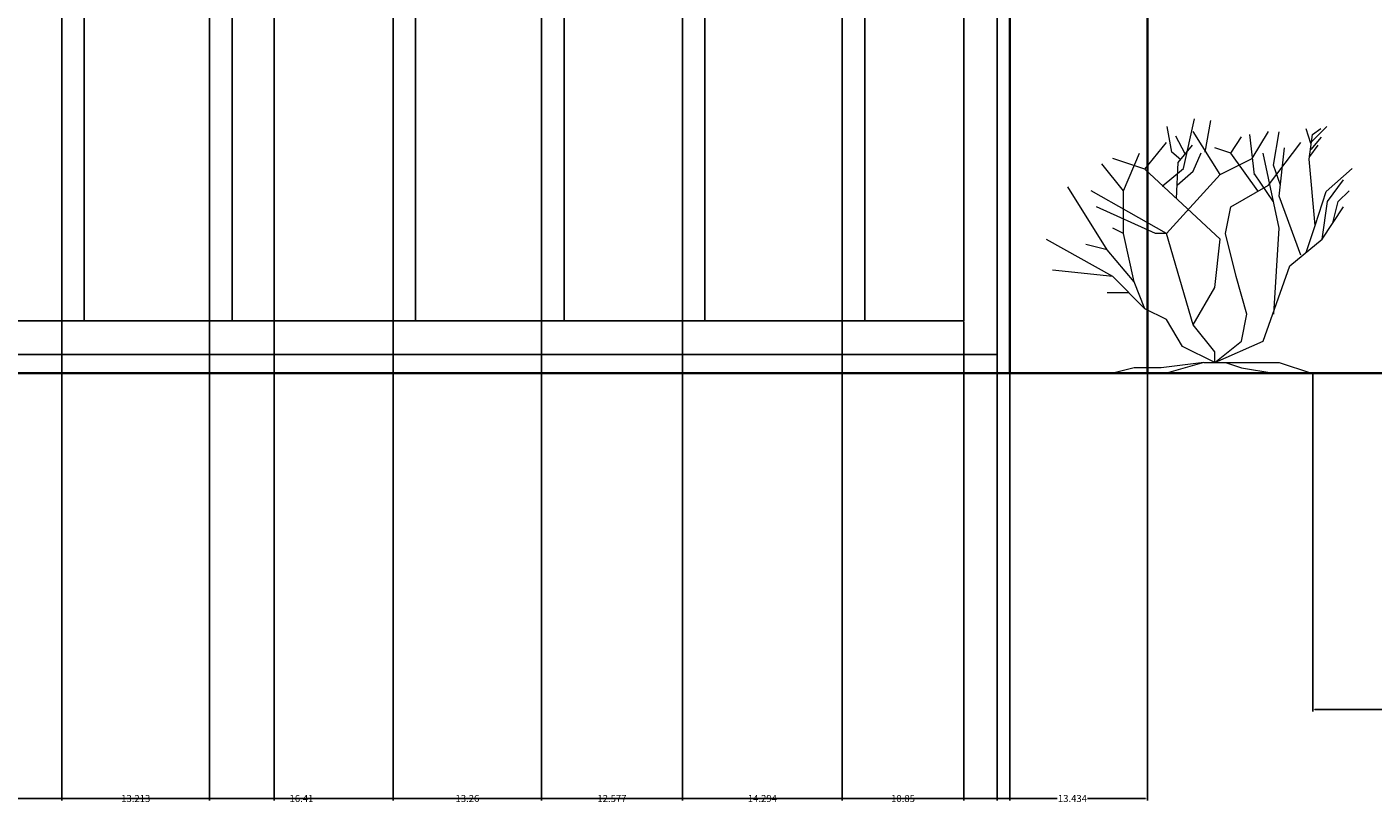
# Model space of a CAD drawing. Units: inches. Extents: x -13 to 809, y 112 to 656.
# Tile 41 of 55: x 521 to 641, y 112 to 181. Entities that reach past the tile are written whole.
import ezdxf

# ---------------------------------------------------------------- set-up
doc = ezdxf.new("R2010")
doc.units = ezdxf.units.IN
doc.header["$MEASUREMENT"] = 0
for name, color, linetype, lineweight in [('A-ANNO-DIMS', 2, 'Continuous', 18), ('A-DOOR', 4, 'Continuous', 25), ('A-ELEV', 7, 'Continuous', 35), ('L-PLNT', 3, 'Continuous', 18)]:
    doc.layers.add(name, color=color, linetype=linetype, lineweight=lineweight)
doc.styles.get("Standard").update_dxf_attribs({"font": 'arial.ttf'})
doc.dimstyles.get("Standard").update_dxf_attribs({"dimtxt": 0.625, "dimasz": 0.18, "dimexe": 0.18, "dimexo": 0.0625, "dimgap": 0.09, "dimtad": 0, "dimtih": 1, "dimtoh": 1, "dimdec": 4, "dimzin": 0, "dimdsep": 46, "dimlunit": 4, "dimtxsty": 'Standard', "dimcen": 0.09, "dimadec": 0, "dimazin": 0, "dimtfac": 1, "dimtdec": 4, "dimtofl": 0, "dimtmove": 0, "dimatfit": 3, "dimfxl": 1, "dimtolj": 1, "dimtzin": 0, "dimarcsym": 0})

# ---------------------------------------------------------------- blocks, each defined once
blk = doc.blocks.new('Shrub - elevation')
for p, q in [((-12.471, 19.775), (-12.898, 22.044)), ((-11.433, 18.289), (-10.457, 22.749)), ((-9.48, 19.775), (-8.992, 22.592)), ((-0.508, 21.888), (-0.081, 20.558)), ((0.041, 20.714), (1.384, 22.044)), ((0.102, 21.34), (0.835, 21.888)), ((-14.88, 18.24), (-12.96, 20.64)), ((-11.28, 19.619), (-12.104, 21.184)), ((-8.16, 17.76), (-10.56, 21.6)), ((-7.2, 19.68), (-6.24, 21.12)), ((-5.086, 17.741), (-5.513, 21.34)), ((-5.28, 19.2), (-3.84, 21.6)), ((-3.84, 16.8), (-0.96, 20.64)), ((-3.377, 18.602), (-2.888, 21.575)), ((-0.203, 19.149), (0.102, 21.34)), ((-0.02, 20.01), (0.896, 21.105)), ((-16.8, 16.32), (-15.36, 19.68)), ((-11.677, 19.071), (-12.471, 19.775)), ((-11.921, 18.836), (-10.64, 20.401)), ((-10.579, 18.054), (-9.846, 19.697)), ((-7.2, 19.68), (-8.64, 20.16)), ((-4.8, 16.32), (-7.2, 19.68)), ((-2.88, 12.96), (-4.32, 19.68)), ((-2.88, 15.84), (-2.4, 20.16)), ((-0.142, 19.384), (0.59, 20.401)), ((-16.8, 16.32), (-18.72, 18.72)), ((-14.88, 18.24), (-17.76, 19.2)), ((-8.16, 12), (-14.88, 18.24)), ((-13.325, 16.724), (-11.433, 18.289)), ((-12.043, 15.628), (-11.921, 18.836)), ((-11.982, 16.802), (-10.579, 18.054)), ((-8.16, 17.76), (-5.28, 19.2)), ((-2.766, 16.802), (-3.377, 18.602)), ((0.346, 13.203), (-0.203, 19.149)), ((1.323, 16.254), (3.642, 18.289)), ((-12.96, 12.48), (-8.16, 17.76)), ((-3.377, 15.315), (-5.086, 17.819)), ((1.44, 15.36), (2.88, 17.28)), ((-18.24, 11.04), (-21.755, 16.655)), ((-12.96, 12.48), (-19.68, 16.32)), ((-16.8, 12.48), (-16.8, 16.32)), ((-7.2, 14.88), (-3.84, 16.8)), ((-0.96, 10.56), (-2.88, 15.84)), ((0.346, 13.203), (1.323, 16.254)), ((2.4, 15.36), (3.36, 16.32)), ((-13.92, 12.48), (-19.2, 14.88)), ((-7.68, 12.48), (-7.2, 14.88)), ((0.96, 12), (1.44, 15.36)), ((0.96, 12), (2.88, 14.88)), ((1.92, 13.44), (2.4, 15.36)), ((-16.8, 12.48), (-17.76, 12.96)), ((-15.84, 8.16), (-16.8, 12.48)), ((-12.96, 12.48), (-13.92, 12.48)), ((-10.56, 4.32), (-12.96, 12.48)), ((-6.72, 8.64), (-7.68, 12.48)), ((-3.36, 5.28), (-2.88, 12.96)), ((-0.48, 10.8), (0.346, 13.203)), ((-17.76, 8.64), (-23.663, 11.961)), ((-18.24, 11.04), (-20.16, 11.52)), ((-15.84, 8.16), (-18.24, 11.04)), ((-8.64, 7.68), (-8.16, 12)), ((-1.92, 9.6), (0.96, 12)), ((-17.76, 8.64), (-23.128, 9.222)), ((-14.88, 5.76), (-17.76, 8.64)), ((-5.76, 5.28), (-6.72, 8.64)), ((-4.32, 2.88), (-1.92, 9.6)), ((-14.88, 5.76), (-15.84, 8.16)), ((-10.56, 4.32), (-8.64, 7.68)), ((-16.32, 7.2), (-18.24, 7.2)), ((-12.96, 4.8), (-14.88, 5.76)), ((-6.24, 2.88), (-5.76, 5.28)), ((-11.52, 2.4), (-12.96, 4.8)), ((-8.64, 1.92), (-10.56, 4.32)), ((-8.64, 0.96), (-4.32, 2.88)), ((-8.64, 0.96), (-6.24, 2.88)), ((-8.64, 0.96), (-11.52, 2.4)), ((-8.64, 0.96), (-8.64, 1.92)), ((-15.84, 0.48), (-17.76, 0)), ((-13.44, 0.48), (-15.84, 0.48)), ((-9.6, 0.96), (-13.44, 0.48)), ((-9.6, 0.96), (-12.96, 0)), ((-9.6, 0.96), (-7.68, 0.96)), ((-8.64, 0.96), (-2.88, 0.96)), ((-7.68, 0.96), (-6.24, 0.48)), ((-6.24, 0.48), (-3.36, 0)), ((-2.88, 0.96), (0, 0))]:
    blk.add_line(p, q)
blk = doc.blocks.new('*D10')
at = {"layer": 'A-ANNO-DIMS', "color": 0, "lineweight": -2, "transparency": 16777216}
for p, q in [((635.78, 150.57), (635.78, 120.28)), ((711.75, 150.57), (711.75, 120.28)), ((635.96, 120.46), (673.23, 120.46)), ((711.57, 120.46), (674.3, 120.46))]:
    blk.add_line(p, q, dxfattribs=at)
at = {"layer": 'A-ANNO-DIMS', "color": 0, "transparency": 16777216}
for points in [[(635.96, 120.49), (635.96, 120.43), (635.78, 120.46)], [(711.57, 120.49), (711.57, 120.43), (711.75, 120.46)]]:
    blk.add_solid(points, dxfattribs=at)
at = {"layer": 'Defpoints', "color": 0, "transparency": 16777216}
for p in [(635.78, 150.63), (711.75, 150.63), (711.75, 120.46)]:
    blk.add_point(p, dxfattribs=at)
at = {"layer": 'A-ANNO-DIMS', "color": 0, "transparency": 16777216, "insert": (673.77, 120.46), "char_height": 0.625, "attachment_point": 5}
blk.add_mtext('\\A1;76', dxfattribs=at)
blk = doc.blocks.new('*D20')
at = {"layer": 'A-ANNO-DIMS', "color": 0, "lineweight": -2, "transparency": 16777216}
for p, q in [((365.94, 210.72), (365.94, 112.34)), ((607.57, 209.81), (607.57, 112.34)), ((366.12, 112.52), (485.36, 112.52)), ((607.39, 112.52), (488.15, 112.52))]:
    blk.add_line(p, q, dxfattribs=at)
at = {"layer": 'A-ANNO-DIMS', "color": 0, "transparency": 16777216}
for points in [[(366.12, 112.55), (366.12, 112.49), (365.94, 112.52)], [(607.39, 112.55), (607.39, 112.49), (607.57, 112.52)]]:
    blk.add_solid(points, dxfattribs=at)
at = {"layer": 'Defpoints', "color": 0, "transparency": 16777216}
for p in [(365.94, 210.78), (607.57, 209.88), (607.57, 112.52)]:
    blk.add_point(p, dxfattribs=at)
at = {"layer": 'A-ANNO-DIMS', "color": 0, "transparency": 16777216, "insert": (486.76, 112.52), "char_height": 0.625, "attachment_point": 5}
blk.add_mtext('\\A1;241.64', dxfattribs=at)
blk = doc.blocks.new('*D21')
at = {"layer": 'A-ANNO-DIMS', "color": 0, "lineweight": -2, "transparency": 16777216}
for p, q in [((607.57, 209.81), (607.57, 112.34)), ((621.01, 150.46), (621.01, 112.34)), ((607.75, 112.52), (612.93, 112.52)), ((620.83, 112.52), (615.65, 112.52))]:
    blk.add_line(p, q, dxfattribs=at)
at = {"layer": 'A-ANNO-DIMS', "color": 0, "transparency": 16777216}
for points in [[(607.75, 112.55), (607.75, 112.49), (607.57, 112.52)], [(620.83, 112.55), (620.83, 112.49), (621.01, 112.52)]]:
    blk.add_solid(points, dxfattribs=at)
at = {"layer": 'Defpoints', "color": 0, "transparency": 16777216}
for p in [(607.57, 209.88), (621.01, 150.52), (621.01, 112.52)]:
    blk.add_point(p, dxfattribs=at)
at = {"layer": 'A-ANNO-DIMS', "color": 0, "transparency": 16777216, "insert": (614.29, 112.52), "char_height": 0.625, "attachment_point": 5}
blk.add_mtext('\\A1;13.434', dxfattribs=at)
blk = doc.blocks.new('*D31')
at = {"layer": 'A-ANNO-DIMS', "color": 0, "lineweight": -2, "transparency": 16777216}
for p, q in [((621.07, 617.78), (807.77, 617.78)), ((807.59, 617.6), (807.59, 384.56)), ((807.59, 150.7), (807.59, 383.74)), ((621.07, 150.52), (807.77, 150.52))]:
    blk.add_line(p, q, dxfattribs=at)
at = {"layer": 'A-ANNO-DIMS', "color": 0, "transparency": 16777216}
for points in [[(807.56, 617.6), (807.62, 617.6), (807.59, 617.78)], [(807.56, 150.7), (807.62, 150.7), (807.59, 150.52)]]:
    blk.add_solid(points, dxfattribs=at)
at = {"layer": 'Defpoints', "color": 0, "transparency": 16777216}
for p in [(621.01, 617.78), (807.59, 617.78), (621.01, 150.52)]:
    blk.add_point(p, dxfattribs=at)
at = {"layer": 'A-ANNO-DIMS', "color": 0, "transparency": 16777216, "insert": (807.59, 384.15), "char_height": 0.625, "attachment_point": 5}
blk.add_mtext('\\A1;467.3', dxfattribs=at)
blk = doc.blocks.new('*D52')
at = {"layer": 'A-ANNO-DIMS', "color": 0, "lineweight": -2, "transparency": 16777216}
for p, q in [((442.18, 288.39), (442.18, 112.34)), ((542.96, 288.39), (542.96, 112.34)), ((442.36, 112.52), (491.21, 112.52)), ((542.78, 112.52), (493.93, 112.52))]:
    blk.add_line(p, q, dxfattribs=at)
at = {"layer": 'A-ANNO-DIMS', "color": 0, "transparency": 16777216}
for points in [[(442.36, 112.55), (442.36, 112.49), (442.18, 112.52)], [(542.78, 112.55), (542.78, 112.49), (542.96, 112.52)]]:
    blk.add_solid(points, dxfattribs=at)
at = {"layer": 'Defpoints', "color": 0, "transparency": 16777216}
for p in [(442.18, 288.45), (542.96, 288.45), (542.96, 112.52)]:
    blk.add_point(p, dxfattribs=at)
at = {"layer": 'A-ANNO-DIMS', "color": 0, "transparency": 16777216, "insert": (492.57, 112.52), "char_height": 0.625, "attachment_point": 5}
blk.add_mtext('\\A1;100.78', dxfattribs=at)
blk = doc.blocks.new('*D129')
at = {"layer": 'A-ANNO-DIMS', "color": 0, "lineweight": -2, "transparency": 16777216}
for p, q in [((607.64, 209.88), (807.77, 209.88)), ((807.59, 209.7), (807.59, 180.61)), ((807.59, 150.7), (807.59, 179.79)), ((608.76, 150.52), (807.77, 150.52))]:
    blk.add_line(p, q, dxfattribs=at)
at = {"layer": 'A-ANNO-DIMS', "color": 0, "transparency": 16777216}
for points in [[(807.56, 209.7), (807.62, 209.7), (807.59, 209.88)], [(807.56, 150.7), (807.62, 150.7), (807.59, 150.52)]]:
    blk.add_solid(points, dxfattribs=at)
at = {"layer": 'Defpoints', "color": 0, "transparency": 16777216}
for p in [(607.57, 209.88), (807.59, 209.88), (608.69, 150.52)]:
    blk.add_point(p, dxfattribs=at)
at = {"layer": 'A-ANNO-DIMS', "color": 0, "transparency": 16777216, "insert": (807.59, 180.2), "char_height": 0.625, "attachment_point": 5}
blk.add_mtext('\\A1;59.36', dxfattribs=at)
blk = doc.blocks.new('*D130')
at = {"layer": 'A-ANNO-DIMS', "color": 0, "lineweight": -2, "transparency": 16777216}
for p, q in [((365.94, 152.15), (365.94, 112.34)), ((608.69, 150.46), (608.69, 112.34)), ((366.12, 112.52), (485.92, 112.52)), ((608.51, 112.52), (488.71, 112.52))]:
    blk.add_line(p, q, dxfattribs=at)
at = {"layer": 'A-ANNO-DIMS', "color": 0, "transparency": 16777216}
for points in [[(366.12, 112.55), (366.12, 112.49), (365.94, 112.52)], [(608.51, 112.55), (608.51, 112.49), (608.69, 112.52)]]:
    blk.add_solid(points, dxfattribs=at)
at = {"layer": 'Defpoints', "color": 0, "transparency": 16777216}
for p in [(365.94, 152.21), (608.69, 150.52), (608.69, 112.52)]:
    blk.add_point(p, dxfattribs=at)
at = {"layer": 'A-ANNO-DIMS', "color": 0, "transparency": 16777216, "insert": (487.32, 112.52), "char_height": 0.625, "attachment_point": 5}
blk.add_mtext('\\A1;242.76', dxfattribs=at)
blk = doc.blocks.new('*D148')
at = {"layer": 'A-ANNO-DIMS', "color": 0, "lineweight": -2, "transparency": 16777216}
for p, q in [((509.9, 155.15), (509.9, 112.34)), ((523.97, 155.15), (523.97, 112.34)), ((510.08, 112.52), (515.82, 112.52)), ((523.79, 112.52), (518.05, 112.52))]:
    blk.add_line(p, q, dxfattribs=at)
at = {"layer": 'A-ANNO-DIMS', "color": 0, "transparency": 16777216}
for points in [[(510.08, 112.55), (510.08, 112.49), (509.9, 112.52)], [(523.79, 112.55), (523.79, 112.49), (523.97, 112.52)]]:
    blk.add_solid(points, dxfattribs=at)
at = {"layer": 'Defpoints', "color": 0, "transparency": 16777216}
for p in [(509.9, 155.21), (523.97, 155.21), (523.97, 112.52)]:
    blk.add_point(p, dxfattribs=at)
at = {"layer": 'A-ANNO-DIMS', "color": 0, "transparency": 16777216, "insert": (516.94, 112.52), "char_height": 0.625, "attachment_point": 5}
blk.add_mtext('\\A1;14.07', dxfattribs=at)
blk = doc.blocks.new('*D149')
at = {"layer": 'A-ANNO-DIMS', "color": 0, "lineweight": -2, "transparency": 16777216}
for p, q in [((523.97, 155.15), (523.97, 112.34)), ((537.18, 155.15), (537.18, 112.34)), ((524.15, 112.52), (529.22, 112.52)), ((537, 112.52), (531.94, 112.52))]:
    blk.add_line(p, q, dxfattribs=at)
at = {"layer": 'A-ANNO-DIMS', "color": 0, "transparency": 16777216}
for points in [[(524.15, 112.55), (524.15, 112.49), (523.97, 112.52)], [(537, 112.55), (537, 112.49), (537.18, 112.52)]]:
    blk.add_solid(points, dxfattribs=at)
at = {"layer": 'Defpoints', "color": 0, "transparency": 16777216}
for p in [(523.97, 155.21), (537.18, 155.21), (537.18, 112.52)]:
    blk.add_point(p, dxfattribs=at)
at = {"layer": 'A-ANNO-DIMS', "color": 0, "transparency": 16777216, "insert": (530.58, 112.52), "char_height": 0.625, "attachment_point": 5}
blk.add_mtext('\\A1;13.213', dxfattribs=at)
blk = doc.blocks.new('*D150')
at = {"layer": 'A-ANNO-DIMS', "color": 0, "lineweight": -2, "transparency": 16777216}
for p, q in [((537.18, 155.15), (537.18, 112.34)), ((553.6, 155.15), (553.6, 112.34)), ((537.36, 112.52), (544.33, 112.52)), ((553.42, 112.52), (546.44, 112.52))]:
    blk.add_line(p, q, dxfattribs=at)
at = {"layer": 'A-ANNO-DIMS', "color": 0, "transparency": 16777216}
for points in [[(537.36, 112.55), (537.36, 112.49), (537.18, 112.52)], [(553.42, 112.55), (553.42, 112.49), (553.6, 112.52)]]:
    blk.add_solid(points, dxfattribs=at)
at = {"layer": 'Defpoints', "color": 0, "transparency": 16777216}
for p in [(537.18, 155.21), (553.6, 155.21), (553.6, 112.52)]:
    blk.add_point(p, dxfattribs=at)
at = {"layer": 'A-ANNO-DIMS', "color": 0, "transparency": 16777216, "insert": (545.39, 112.52), "char_height": 0.625, "attachment_point": 5}
blk.add_mtext('\\A1;16.41', dxfattribs=at)
blk = doc.blocks.new('*D151')
at = {"layer": 'A-ANNO-DIMS', "color": 0, "lineweight": -2, "transparency": 16777216}
for p, q in [((553.6, 155.15), (553.6, 112.34)), ((566.85, 155.15), (566.85, 112.34)), ((553.78, 112.52), (559.11, 112.52)), ((566.67, 112.52), (561.34, 112.52))]:
    blk.add_line(p, q, dxfattribs=at)
at = {"layer": 'A-ANNO-DIMS', "color": 0, "transparency": 16777216}
for points in [[(553.78, 112.55), (553.78, 112.49), (553.6, 112.52)], [(566.67, 112.55), (566.67, 112.49), (566.85, 112.52)]]:
    blk.add_solid(points, dxfattribs=at)
at = {"layer": 'Defpoints', "color": 0, "transparency": 16777216}
for p in [(553.6, 155.21), (566.85, 155.21), (566.85, 112.52)]:
    blk.add_point(p, dxfattribs=at)
at = {"layer": 'A-ANNO-DIMS', "color": 0, "transparency": 16777216, "insert": (560.22, 112.52), "char_height": 0.625, "attachment_point": 5}
blk.add_mtext('\\A1;13.26', dxfattribs=at)
blk = doc.blocks.new('*D152')
at = {"layer": 'A-ANNO-DIMS', "color": 0, "lineweight": -2, "transparency": 16777216}
for p, q in [((566.85, 155.15), (566.85, 112.34)), ((579.43, 155.15), (579.43, 112.34)), ((567.03, 112.52), (571.78, 112.52)), ((579.25, 112.52), (574.5, 112.52))]:
    blk.add_line(p, q, dxfattribs=at)
at = {"layer": 'A-ANNO-DIMS', "color": 0, "transparency": 16777216}
for points in [[(567.03, 112.55), (567.03, 112.49), (566.85, 112.52)], [(579.25, 112.55), (579.25, 112.49), (579.43, 112.52)]]:
    blk.add_solid(points, dxfattribs=at)
at = {"layer": 'Defpoints', "color": 0, "transparency": 16777216}
for p in [(566.85, 155.21), (579.43, 155.21), (579.43, 112.52)]:
    blk.add_point(p, dxfattribs=at)
at = {"layer": 'A-ANNO-DIMS', "color": 0, "transparency": 16777216, "insert": (573.14, 112.52), "char_height": 0.625, "attachment_point": 5}
blk.add_mtext('\\A1;12.577', dxfattribs=at)
blk = doc.blocks.new('*D153')
at = {"layer": 'A-ANNO-DIMS', "color": 0, "lineweight": -2, "transparency": 16777216}
for p, q in [((579.43, 155.15), (579.43, 112.34)), ((593.72, 155.15), (593.72, 112.34)), ((579.61, 112.52), (585.22, 112.52)), ((593.54, 112.52), (587.93, 112.52))]:
    blk.add_line(p, q, dxfattribs=at)
at = {"layer": 'A-ANNO-DIMS', "color": 0, "transparency": 16777216}
for points in [[(579.61, 112.55), (579.61, 112.49), (579.43, 112.52)], [(593.54, 112.55), (593.54, 112.49), (593.72, 112.52)]]:
    blk.add_solid(points, dxfattribs=at)
at = {"layer": 'Defpoints', "color": 0, "transparency": 16777216}
for p in [(579.43, 155.21), (593.72, 155.21), (593.72, 112.52)]:
    blk.add_point(p, dxfattribs=at)
at = {"layer": 'A-ANNO-DIMS', "color": 0, "transparency": 16777216, "insert": (586.58, 112.52), "char_height": 0.625, "attachment_point": 5}
blk.add_mtext('\\A1;14.294', dxfattribs=at)
blk = doc.blocks.new('*D154')
at = {"layer": 'A-ANNO-DIMS', "color": 0, "lineweight": -2, "transparency": 16777216}
for p, q in [((593.72, 155.15), (593.72, 112.34)), ((604.57, 155.15), (604.57, 112.34)), ((593.9, 112.52), (598.03, 112.52)), ((604.39, 112.52), (600.27, 112.52))]:
    blk.add_line(p, q, dxfattribs=at)
at = {"layer": 'A-ANNO-DIMS', "color": 0, "transparency": 16777216}
for points in [[(593.9, 112.55), (593.9, 112.49), (593.72, 112.52)], [(604.39, 112.55), (604.39, 112.49), (604.57, 112.52)]]:
    blk.add_solid(points, dxfattribs=at)
at = {"layer": 'Defpoints', "color": 0, "transparency": 16777216}
for p in [(593.72, 155.21), (604.57, 155.21), (604.57, 112.52)]:
    blk.add_point(p, dxfattribs=at)
at = {"layer": 'A-ANNO-DIMS', "color": 0, "transparency": 16777216, "insert": (599.15, 112.52), "char_height": 0.625, "attachment_point": 5}
blk.add_mtext('\\A1;10.85', dxfattribs=at)

msp = doc.modelspace()

# ---------------------------------------------------------------- linework, layer by layer
at = {"layer": 'A-DOOR'}
for p, q in [((523.9709, 207.19), (523.9709, 155.2141)), ((525.9709, 207.1825), (525.9709, 155.2141)), ((537.1843, 207.1403), (537.1843, 155.2141)), ((539.1843, 207.1328), (539.1843, 155.2141)), ((553.5951, 207.0785), (553.5951, 155.2141)), ((555.5951, 207.071), (555.5951, 155.2141)), ((566.8541, 207.0286), (566.8541, 155.2141)), ((568.8541, 207.0211), (568.8541, 155.2141)), ((579.4311, 206.9813), (579.4311, 155.2141)), ((581.4311, 206.9737), (581.4311, 155.2141)), ((593.7248, 206.9274), (593.7248, 155.2141)), ((595.7248, 206.9199), (595.7248, 155.2141))]:
    msp.add_line(p, q, dxfattribs=at)
for points in [[(365.9383, 210.7849), (607.5741, 209.8753), (607.5741, 152.2141), (365.9383, 152.2141)], [(368.9383, 207.7736), (604.5741, 206.8866), (604.5741, 155.2141), (368.9383, 155.2141)]]:
    msp.add_lwpolyline(points, close=True, dxfattribs=at)
at = {"layer": 'A-ELEV'}
for p, q in [((608.694, 209.8635), (608.694, 150.5199)), ((621.008, 209.8635), (621.008, 150.5199)), ((109.5888, 150.5199), (649.5888, 150.5199))]:
    msp.add_line(p, q, dxfattribs=at)

# ---------------------------------------------------------------- block references
at = {"layer": 'L-PLNT'}
msp.add_blockref('Shrub - elevation', (635.6459, 150.5199), dxfattribs=at)

# ---------------------------------------------------------------- dimensions: what is measured, and where the dimension line sits
at = {"layer": 'A-ANNO-DIMS'}
for base, p1, p2, override, picture, middle in [((807.5888, 617.7828), (621.008, 150.5199), (621.008, 617.7828), {"dimdec": 1, "dimlfac": 1, "dimrnd": 0, "dimzin": 0, "dimdsep": 46, "dimlunit": 2}, '*D31', (807.5888, 384.1514)), ((807.5888, 209.8753), (608.694, 150.5199), (607.5741, 209.8753), {"dimdec": 2, "dimlfac": 1, "dimrnd": 0, "dimzin": 0, "dimdsep": 46, "dimlunit": 2}, '*D129', (807.5888, 180.1976))]:
    dim = msp.add_linear_dim(base=base, p1=p1, p2=p2, angle=90, dimstyle='Standard', override=override, dxfattribs=at)
    dim.commit()
    dim.dimension.update_dxf_attribs({"geometry": picture, "text_midpoint": middle})
for base, p1, p2, override, picture, middle in [((542.9617, 112.5199), (442.1845, 288.4508), (542.9617, 288.4508), {"dimdec": 2, "dimlfac": 1, "dimrnd": 0, "dimzin": 0, "dimdsep": 46, "dimlunit": 2}, '*D52', (492.5731, 112.5199)), ((607.5741, 112.5199), (365.9383, 210.7849), (607.5741, 209.8753), {"dimdec": 2, "dimlfac": 1, "dimrnd": 0, "dimzin": 0, "dimdsep": 46, "dimlunit": 2}, '*D20', (486.7562, 112.5199)), ((621.008, 112.5199), (607.5741, 209.8753), (621.008, 150.5199), {"dimdec": 3, "dimlfac": 1, "dimrnd": 0, "dimzin": 0, "dimdsep": 46, "dimlunit": 2}, '*D21', (614.2911, 112.5199)), ((523.9709, 112.5199), (509.8998, 155.2141), (523.9709, 155.2141), {"dimdec": 2, "dimlfac": 1, "dimrnd": 0, "dimzin": 0, "dimdsep": 46, "dimlunit": 2}, '*D148', (516.9353, 112.5199)), ((537.1843, 112.5199), (523.9709, 155.2141), (537.1843, 155.2141), {"dimdec": 3, "dimlfac": 1, "dimrnd": 0, "dimzin": 0, "dimdsep": 46, "dimlunit": 2}, '*D149', (530.5776, 112.5199)), ((553.5951, 112.5199), (537.1843, 155.2141), (553.5951, 155.2141), {"dimdec": 2, "dimlfac": 1, "dimrnd": 0, "dimzin": 0, "dimdsep": 46, "dimlunit": 2}, '*D150', (545.3897, 112.5199)), ((566.8541, 112.5199), (553.5951, 155.2141), (566.8541, 155.2141), {"dimdec": 2, "dimlfac": 1, "dimrnd": 0, "dimzin": 0, "dimdsep": 46, "dimlunit": 2}, '*D151', (560.2246, 112.5199)), ((579.4311, 112.5199), (566.8541, 155.2141), (579.4311, 155.2141), {"dimdec": 3, "dimlfac": 1, "dimrnd": 0, "dimzin": 0, "dimdsep": 46, "dimlunit": 2}, '*D152', (573.1426, 112.5199)), ((593.7248, 112.5199), (579.4311, 155.2141), (593.7248, 155.2141), {"dimdec": 3, "dimlfac": 1, "dimrnd": 0, "dimzin": 0, "dimdsep": 46, "dimlunit": 2}, '*D153', (586.578, 112.5199)), ((604.5741, 112.5199), (593.7248, 155.2141), (604.5741, 155.2141), {"dimdec": 2, "dimlfac": 1, "dimrnd": 0, "dimzin": 0, "dimdsep": 46, "dimlunit": 2}, '*D154', (599.1494, 112.5199)), ((608.694, 112.5199), (365.9383, 152.2141), (608.694, 150.5199), {"dimdec": 2, "dimlfac": 1, "dimrnd": 0, "dimzin": 0, "dimdsep": 46, "dimlunit": 2}, '*D130', (487.3161, 112.5199)), ((711.7495, 120.4592), (635.7844, 150.6343), (711.7495, 150.6343), {"dimdec": 0, "dimlfac": 1, "dimrnd": 0, "dimzin": 0, "dimdsep": 46, "dimlunit": 2}, '*D10', (673.7669, 120.4592))]:
    dim = msp.add_linear_dim(base=base, p1=p1, p2=p2, dimstyle='Standard', override=override, dxfattribs=at)
    dim.commit()
    dim.dimension.update_dxf_attribs({"geometry": picture, "text_midpoint": middle})

doc.saveas('drawing.dxf')
